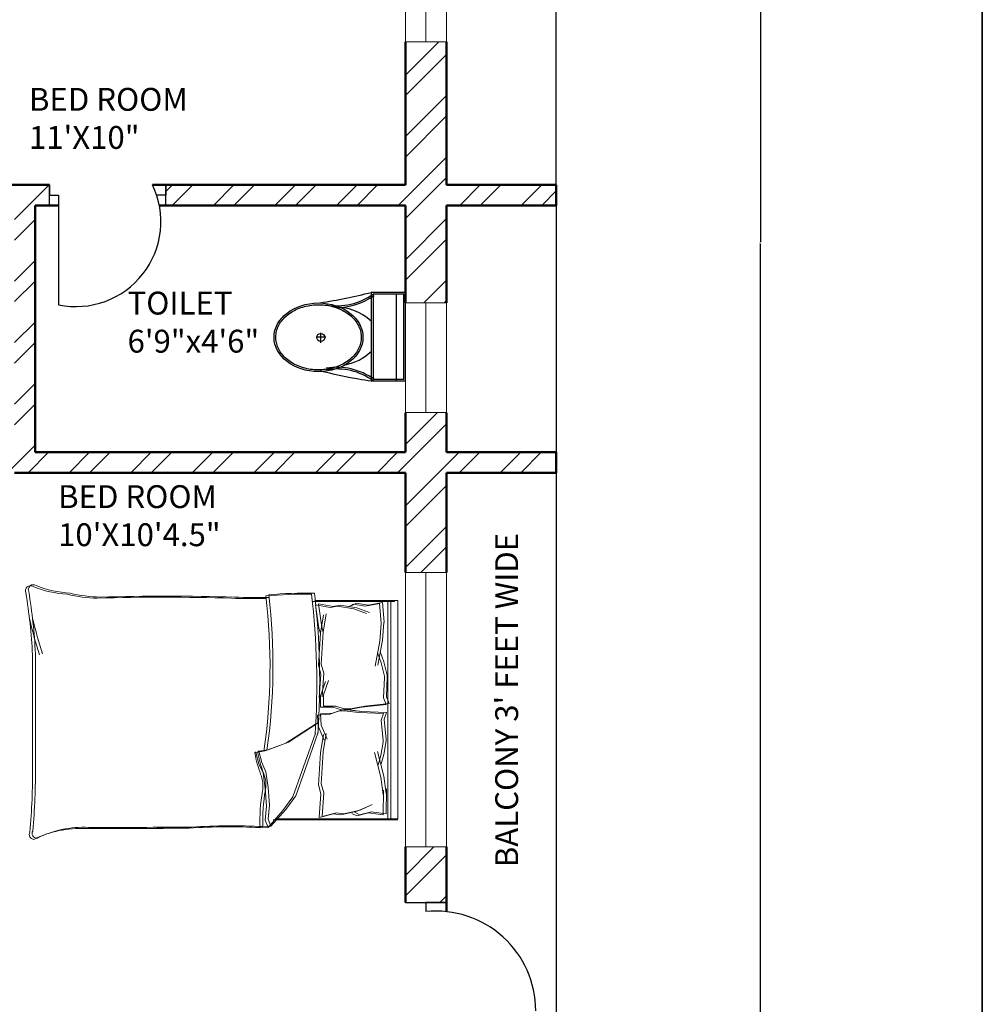
# Model space of a CAD drawing. Units: inches. Extents: x 1980 to 2738, y 1471 to 2568.
# Tile 21 of 22: x 2528 to 2738, y 2112 to 2328. Entities that reach past the tile are written whole.
import ezdxf

# ---------------------------------------------------------------- set-up
doc = ezdxf.new("R2010")
doc.units = ezdxf.units.IN
for name, color, linetype, lineweight in [('A-ANNO-DIMS', 2, 'Continuous', 18), ('A-ANNO-TTLB', 7, 'Continuous', 35), ('A-AREA-IDEN', 7, 'Continuous', 18), ('A-DOOR', 31, 'Continuous', 25), ('A-FLOR-BALC', 7, 'Continuous', 25), ('A-FLOR-FIXT', 8, 'Continuous', 25), ('A-FURN', 8, 'Continuous', 18), ('A-GLAZ', 141, 'Continuous', 18), ('A-WALL', 7, 'Continuous', 50)]:
    doc.layers.add(name, color=color, linetype=linetype, lineweight=lineweight)
doc.layers.add('A-WALL-PATT', color=9, linetype='Continuous', lineweight=13, true_color=0xd19cc7)
doc.styles.get("Standard").update_dxf_attribs({"font": 'arial.ttf'})
doc.dimstyles.get("Standard").update_dxf_attribs({"dimtxt": 0.18, "dimasz": 0.18, "dimexe": 0.18, "dimexo": 0.0625, "dimgap": 0.09, "dimtad": 0, "dimtih": 1, "dimtoh": 1, "dimdec": 4, "dimzin": 0, "dimdsep": 46, "dimtxsty": 'Standard', "dimcen": 0.09, "dimadec": 0, "dimazin": 0, "dimtfac": 1, "dimtdec": 4, "dimtofl": 0, "dimtmove": 0, "dimatfit": 3, "dimfxl": 1, "dimtolj": 1, "dimtzin": 0, "dimarcsym": 0})

# ---------------------------------------------------------------- blocks, each defined once
blk = doc.blocks.new('A$C31115884')
for p, q in [((257.5, 466.4), (257.5, 523.2)), ((283.1, 497.7), (223.4, 497.7)), ((0, 200), (0, 0)), ((520, 200), (0, 200)), ((10, 190), (10, 10)), ((510, 190), (10, 190)), ((510, 10), (510, 190)), ((520, 0), (520, 200)), ((510, 54.5), (0, 54.5)), ((10, 10), (510, 10)), ((0, 0), (520, 0))]:
    blk.add_line(p, q)
blk.add_circle((255.6, 496.4), 23.6)
for centre, radius, start, end in [((2777.7, -204.6), 2807, 165.4549, 171.71327), ((-294.5, 403.3), 364.7, 324.20913, 9.34987), ((-294.5, 403.3), 374.7, 324.20913, 9.34987), ((805.8, 403.3), 364.7, 170.65013, 215.79087), ((3237, 905), 2807, 188.28673, 194.5451), ((139.5, 406.2), 293.5, 315.84364, 2.65635), ((805.8, 403.3), 374.7, 179.20365, 215.79087), ((383.6, 406.2), 293.5, 190.27735, 224.15636)]:
    blk.add_arc(centre, radius, start, end)
blk.add_ellipse((256.2, 509.9), major_axis=(0, -260.7), ratio=0.772727)
blk.add_open_spline([(256.2, 259.2), (263.1, 259.2), (270, 259.7), (287.8, 262.3), (298.7, 265.1), (319.9, 273.1), (330.2, 278.4), (350.1, 291.1), (359.7, 298.7), (377.7, 315.9), (386.2, 325.5), (401.7, 346.6), (408.8, 358.1), (421.3, 382.5), (426.8, 395.5), (435.9, 422.4), (439.5, 436.4), (444.8, 465.1), (446.5, 479.7), (447.9, 509.2), (447.6, 524), (445, 553.3), (442.7, 567.8), (436.3, 596), (432.1, 609.7), (421.9, 636), (416, 648.6), (402.5, 672.1), (395, 683), (378.6, 703), (369.8, 712.1), (351.1, 728), (341.3, 734.8), (320.9, 746.2), (310.4, 750.7), (288.9, 757.3), (278, 759.4), (256, 761), (245, 760.6), (223.1, 757.2), (212.3, 754.3), (191.1, 746.1), (180.8, 740.7), (160.9, 727.8), (151.4, 720.1), (133.5, 702.7), (125.1, 693), (109.6, 671.7), (102.6, 660.2), (90.2, 635.7), (84.9, 622.7), (76, 595.6), (72.4, 581.6), (67.2, 552.9), (65.6, 538.2), (64.4, 508.8), (64.8, 494), (67.5, 464.7), (69.9, 450.2), (76.6, 422), (80.8, 408.3), (91.1, 382.2), (97.2, 369.7), (110.8, 346.3), (118.4, 335.4), (134.8, 315.6), (143.7, 306.7), (162.4, 290.9), (172.3, 284.2), (192.8, 273), (203.3, 268.6), (224.8, 262.2), (235.8, 260.2), (249.9, 259.3), (253, 259.2), (256.2, 259.2)], degree=3, knots=[0, 0, 0, 0, 0.110105, 0.110105, 0.285049, 0.285049, 0.459994, 0.459994, 0.634938, 0.634938, 0.809882, 0.809882, 0.984827, 0.984827, 1.159771, 1.159771, 1.334715, 1.334715, 1.50966, 1.50966, 1.684604, 1.684604, 1.859549, 1.859549, 2.034493, 2.034493, 2.209437, 2.209437, 2.384382, 2.384382, 2.559326, 2.559326, 2.73427, 2.73427, 2.909215, 2.909215, 3.084159, 3.084159, 3.259103, 3.259103, 3.434048, 3.434048, 3.608992, 3.608992, 3.783936, 3.783936, 3.958881, 3.958881, 4.133825, 4.133825, 4.30877, 4.30877, 4.483714, 4.483714, 4.658658, 4.658658, 4.833603, 4.833603, 5.008547, 5.008547, 5.183491, 5.183491, 5.358436, 5.358436, 5.53338, 5.53338, 5.708324, 5.708324, 5.883269, 5.883269, 6.058213, 6.058213, 6.233158, 6.233158, 6.283185, 6.283185, 6.283185, 6.283185])
blk = doc.blocks.new('BED-DOUBLE')
for p, q in [((27.75, 52.87), (24.5, 49.16)), ((27.75, 52.87), (24.5, 49.16)), ((28.38, 53.1), (25.13, 49.39)), ((28.38, 53.1), (25.13, 49.39)), ((29.49, 52.95), (27.75, 52.87, 3.87)), ((29.49, 52.95), (27.75, 52.87, 3.87)), ((28.36, 51.33), (27.75, 52.87)), ((28.36, 51.33), (27.75, 52.87)), ((30.13, 53.18), (28.38, 53.1, 3.87)), ((30.13, 53.18), (28.38, 53.1, 3.87)), ((29, 51.56), (28.38, 53.1)), ((29, 51.56), (28.38, 53.1)), ((0, 51.49), (0.64, 51.49)), ((0, 51.27), (26.61, 51.27)), ((0, 51.27), (26.61, 51.27)), ((0, 51.27), (0, 3.48)), ((0.64, 51.49), (27.25, 51.49)), ((0.64, 51.49), (27.25, 51.49)), ((1.53, 3.48), (1.53, 51.27)), ((1.53, 3.48), (1.53, 51.27)), ((2.17, 3.7), (2.17, 51.49)), ((2.17, 3.7), (2.17, 51.49)), ((2.56, 50.11), (2.46, 44.71)), ((2.56, 50.11), (2.46, 44.71)), ((2.56, 50.11), (5.77, 49.73)), ((2.56, 50.11), (5.77, 49.73)), ((3.2, 50.34), (3.1, 44.94)), ((3.2, 50.34), (3.1, 44.94)), ((3.2, 50.34), (6.41, 49.96)), ((3.2, 50.34), (6.41, 49.96)), ((5.77, 49.73), (8.34, 50.33)), ((5.77, 49.73), (8.34, 50.33)), ((6.41, 49.96), (8.98, 50.56)), ((6.41, 49.96), (8.98, 50.56)), ((11.83, 50.11), (8.26, 49.31)), ((11.83, 50.11), (8.26, 49.31)), ((8.34, 50.33), (9.38, 49.81)), ((8.34, 50.33), (9.38, 49.81)), ((12.47, 50.34), (8.9, 49.54)), ((12.47, 50.34), (8.9, 49.54)), ((8.98, 50.56), (10.02, 50.04)), ((8.98, 50.56), (10.02, 50.04)), ((13.43, 49.92), (11.83, 50.11)), ((13.43, 49.92), (11.83, 50.11)), ((14.07, 50.15), (12.47, 50.34)), ((14.07, 50.15), (12.47, 50.34)), ((16.57, 50.7), (13.43, 49.92)), ((16.57, 50.7), (13.43, 49.92)), ((17.21, 50.93), (14.07, 50.15)), ((17.21, 50.93), (14.07, 50.15)), ((16.17, 45.57), (16.57, 50.7)), ((16.17, 45.57), (16.57, 50.7)), ((16.81, 45.8), (17.21, 50.93)), ((16.81, 45.79), (17.21, 50.93)), ((28.06, 48.23), (28.36, 51.33)), ((28.06, 48.23), (28.36, 51.33)), ((28.69, 48.46), (29, 51.56)), ((28.69, 48.46), (29, 51.56)), ((8.26, 49.31), (5.58, 48.13)), ((8.26, 49.31), (5.58, 48.13)), ((8.9, 49.54), (6.22, 48.36)), ((8.9, 49.54), (6.22, 48.36)), ((24.5, 49.16), (22.33, 46.22)), ((24.5, 49.16), (22.33, 46.22)), ((25.13, 49.39), (22.97, 46.45)), ((25.13, 49.39), (22.97, 46.45)), ((28.36, 44.36), (28.06, 48.23)), ((28.36, 44.36), (28.06, 48.23)), ((29, 44.59), (28.69, 48.46)), ((29, 44.59), (28.69, 48.46)), ((2.46, 44.71), (2.54, 45.71)), ((2.46, 44.71), (2.54, 45.71)), ((2.54, 45.71), (3.07, 41.91)), ((2.54, 45.71), (3.07, 41.91)), ((3.1, 44.94), (3.18, 45.94)), ((3.1, 44.94), (3.18, 45.94)), ((3.18, 45.94), (3.71, 42.14)), ((3.18, 45.94), (3.71, 42.14)), ((16.73, 43.61), (16.17, 45.57)), ((16.73, 43.61), (16.17, 45.57)), ((17.37, 43.83), (16.81, 45.8)), ((17.37, 43.83), (16.81, 45.79)), ((22.33, 46.22), (20.32, 40.64)), ((22.33, 46.22), (20.32, 40.64)), ((22.97, 46.45), (20.96, 40.87)), ((22.97, 46.45), (20.96, 40.87)), ((16.29, 36.6), (16.73, 43.61)), ((16.29, 36.6), (16.73, 43.61)), ((16.93, 36.82), (17.37, 43.83)), ((16.93, 36.82), (17.37, 43.83)), ((28.83, 40.95), (28.36, 44.36)), ((28.83, 40.95), (28.36, 44.36)), ((29.47, 41.18), (29, 44.59)), ((29.47, 41.18), (29, 44.59)), ((3.07, 41.91), (4.42, 36.5)), ((3.07, 41.91), (4.42, 36.5)), ((3.71, 42.14), (5.06, 36.72)), ((3.71, 42.14), (5.06, 36.72)), ((29.76, 38.94), (28.83, 40.95)), ((29.76, 38.94), (28.83, 40.95)), ((30.4, 39.17), (29.47, 41.18)), ((30.4, 39.17), (29.47, 41.18)), ((3.67, 39.2), (3.08, 37.14)), ((3.67, 39.2), (3.08, 37.14)), ((4.31, 39.43), (3.72, 37.36)), ((4.31, 39.43), (3.72, 37.36)), ((20.32, 40.64), (17.38, 32.31)), ((20.32, 40.64), (17.38, 32.31)), ((20.96, 40.87), (18.02, 32.53)), ((20.96, 40.87), (18.02, 32.53)), ((30.38, 36.46), (29.76, 38.94)), ((30.38, 36.46), (29.76, 38.94)), ((31.02, 36.69), (30.4, 39.17)), ((31.02, 36.69), (30.4, 39.17)), ((79.24, 15.06), (79.24, 39.68)), ((79.24, 15.06), (79.24, 39.68)), ((79.88, 15.29), (79.88, 39.91)), ((79.88, 15.29), (79.88, 39.91)), ((3.08, 37.14), (2.54, 34.2)), ((3.08, 37.14), (2.54, 34.2)), ((3.72, 37.36), (3.18, 34.43)), ((3.72, 37.36), (3.18, 34.43)), ((16.27, 32.79), (16.93, 36.82)), ((16.27, 32.79), (16.93, 36.82)), ((29, 36.38), (31.02, 36.69)), ((29, 36.38), (31.02, 36.69)), ((15.63, 32.56), (16.29, 36.6)), ((15.63, 32.56), (16.29, 36.6)), ((18.02, 30.49), (24.52, 34.68)), ((18.02, 30.49), (24.52, 34.68)), ((23.88, 34.45), (28.36, 36.15)), ((23.88, 34.45), (28.36, 36.15)), ((24.52, 34.68), (29, 36.38)), ((24.52, 34.68), (29, 36.38)), ((28.36, 36.15), (30.38, 36.46)), ((28.36, 36.15), (30.38, 36.46)), ((2.54, 34.2), (2.56, 33.88)), ((2.54, 34.2), (2.56, 33.88)), ((2.56, 33.88), (2.98, 29.46)), ((2.56, 33.88), (2.98, 29.46)), ((3.18, 34.43), (3.2, 34.11)), ((3.18, 34.43), (3.2, 34.11)), ((3.2, 34.11), (3.62, 29.68)), ((3.2, 34.11), (3.62, 29.68)), ((16.74, 30.75), (15.45, 33.82)), ((16.74, 30.75), (15.45, 33.82)), ((17.38, 30.98), (16.09, 34.05)), ((17.38, 30.98), (16.09, 34.05)), ((17.38, 30.26), (23.88, 34.45)), ((17.38, 30.26), (23.88, 34.45)), ((16.89, 28.3), (16.74, 30.75)), ((16.89, 28.3), (16.74, 30.75)), ((17.53, 28.53), (17.38, 30.98)), ((17.53, 28.53), (17.38, 30.98)), ((2.98, 29.46), (2.49, 27.98)), ((2.98, 29.46), (2.49, 27.98)), ((3.62, 29.68), (3.13, 28.21)), ((3.62, 29.68), (3.13, 28.21)), ((3.13, 28.21), (8.51, 27.96)), ((3.13, 28.21), (8.51, 27.96)), ((12.38, 27.44), (14.22, 28.13)), ((12.38, 27.44), (14.22, 28.13)), ((13.02, 27.66), (14.86, 28.36)), ((13.02, 27.66), (14.86, 28.36)), ((14.22, 28.13), (16.89, 28.3)), ((14.22, 28.13), (16.89, 28.3)), ((14.86, 28.36), (17.53, 28.53)), ((14.86, 28.36), (17.53, 28.53)), ((1.87, 25.98), (7.22, 26.56)), ((1.87, 25.98), (7.22, 26.56)), ((2.45, 24.54), (1.87, 25.98)), ((2.45, 24.54), (1.87, 25.98)), ((2.49, 27.98), (7.87, 27.73)), ((2.49, 27.98), (7.87, 27.73)), ((2.51, 26.21), (7.86, 26.79)), ((2.51, 26.21), (7.86, 26.79)), ((3.09, 24.77), (2.51, 26.21)), ((3.09, 24.77), (2.51, 26.21)), ((7.22, 26.56), (10.4, 27.14)), ((7.22, 26.56), (10.4, 27.14)), ((7.86, 26.79), (11.04, 27.37)), ((7.86, 26.79), (11.04, 27.37)), ((7.87, 27.73), (11.08, 27.36)), ((7.87, 27.73), (11.08, 27.35)), ((8.51, 27.96), (11.72, 27.58)), ((8.51, 27.96), (11.72, 27.58)), ((10.4, 27.14), (11.7, 27.14)), ((10.4, 27.14), (11.7, 27.14)), ((11.04, 27.37), (12.34, 27.37)), ((11.04, 27.37), (12.34, 27.37)), ((11.08, 27.36), (12.38, 27.44)), ((11.08, 27.35), (12.38, 27.44)), ((11.7, 27.14), (13.58, 26.56)), ((11.7, 27.14), (13.58, 26.56)), ((11.72, 27.58), (13.02, 27.66)), ((11.72, 27.58), (13.02, 27.66)), ((12.34, 27.37), (14.22, 26.79)), ((12.34, 27.37), (14.22, 26.79)), ((13.58, 26.56), (16.26, 26.56)), ((13.58, 26.56), (16.26, 26.56)), ((14.22, 26.79), (16.9, 26.79)), ((14.22, 26.79), (16.9, 26.79)), ((16.26, 26.56), (16.26, 24.1)), ((16.26, 26.56), (16.26, 24.1)), ((16.9, 26.79), (16.9, 24.33)), ((16.9, 26.79), (16.9, 24.33)), ((2.3, 20.09), (2.45, 24.54)), ((2.3, 20.09), (2.45, 24.54)), ((2.94, 20.32), (3.09, 24.77)), ((2.94, 20.32), (3.09, 24.77)), ((16.26, 24.1), (15.17, 20.96)), ((16.26, 24.1), (15.17, 20.96)), ((16.9, 24.33), (15.81, 21.19)), ((16.9, 24.33), (15.81, 21.19)), ((16.17, 19.38), (16.57, 24.52)), ((16.17, 19.38), (16.57, 24.52)), ((16.81, 19.61), (17.21, 24.74)), ((16.81, 19.61), (17.21, 24.74)), ((2.3, 19.77), (2.3, 20.09)), ((2.3, 19.77), (2.3, 20.09)), ((3.03, 16.88), (2.3, 19.77)), ((3.03, 16.88), (2.3, 19.77)), ((2.94, 20), (2.94, 20.32)), ((2.94, 20), (2.94, 20.32)), ((3.67, 17.11), (2.94, 20)), ((3.67, 17.11), (2.94, 20)), ((17.37, 17.65), (16.81, 19.61)), ((17.37, 17.65), (16.81, 19.61)), ((3.32, 12.11), (4.33, 17.6)), ((3.32, 12.11), (4.33, 17.6)), ((3.96, 12.34), (4.97, 17.83)), ((3.96, 12.34), (4.97, 17.83)), ((16.73, 17.42), (16.17, 19.38)), ((16.73, 17.42), (16.17, 19.38)), ((16.29, 10.41), (16.73, 17.42)), ((16.29, 10.41), (16.73, 17.42)), ((16.93, 10.64), (17.37, 17.65)), ((16.93, 10.64), (17.37, 17.65)), ((3.75, 14.86), (3.03, 16.88)), ((3.75, 14.85), (3.03, 16.88)), ((4.39, 15.08), (3.67, 17.11)), ((4.39, 15.08), (3.67, 17.11)), ((3.03, 8.29), (3.32, 12.11)), ((3.03, 8.28), (3.32, 12.11)), ((3.67, 8.51), (3.96, 12.34)), ((3.67, 8.51), (3.96, 12.34)), ((15.63, 6.38), (16.29, 10.41)), ((15.63, 6.38), (16.29, 10.41)), ((16.27, 6.61), (16.93, 10.64)), ((16.27, 6.61), (16.93, 10.64)), ((16.29, 10.41), (16.62, 9.28)), ((16.29, 10.41), (16.62, 9.28)), ((16.62, 9.28), (17.34, 4.18)), ((16.62, 9.28), (17.34, 4.18)), ((16.93, 10.64), (17.26, 9.51)), ((16.93, 10.64), (17.26, 9.51)), ((17.26, 9.51), (17.98, 4.41)), ((17.26, 9.51), (17.98, 4.41)), ((3.01, 8.18), (3.03, 8.29)), ((3.01, 8.18), (3.03, 8.28)), ((3.34, 3.9), (3.01, 8.18)), ((3.34, 3.9), (3.01, 8.18)), ((3.65, 8.41), (3.67, 8.51)), ((3.65, 8.41), (3.67, 8.51)), ((3.98, 4.13), (3.65, 8.41)), ((3.98, 4.13), (3.65, 8.41)), ((3.32, 3.89), (6.5, 4.47)), ((3.32, 3.89), (6.5, 4.47)), ((3.96, 4.12), (7.14, 4.7)), ((3.96, 4.12), (7.14, 4.7)), ((8.95, 5.05), (6.21, 6.06)), ((8.95, 5.05), (6.21, 6.06)), ((6.5, 4.47), (9.1, 4.04)), ((6.5, 4.47), (9.1, 4.04)), ((9.59, 5.28), (6.85, 6.29)), ((9.59, 5.28), (6.85, 6.29)), ((7.14, 4.7), (9.74, 4.27)), ((7.14, 4.7), (9.74, 4.27)), ((12.57, 4.47), (8.95, 5.05)), ((12.57, 4.47), (8.95, 5.05)), ((9.1, 4.04), (10.11, 4.62)), ((9.1, 4.04), (10.11, 4.62)), ((13.21, 4.7), (9.59, 5.28)), ((13.21, 4.7), (9.59, 5.28)), ((9.74, 4.27), (10.75, 4.85)), ((9.74, 4.27), (10.75, 4.85)), ((14.16, 4.76), (12.57, 4.47)), ((14.16, 4.76), (12.57, 4.47)), ((14.8, 4.99), (13.21, 4.7)), ((14.8, 4.99), (13.21, 4.7)), ((17.34, 4.18), (14.16, 4.76)), ((17.34, 4.18), (14.16, 4.76)), ((17.98, 4.41), (14.8, 4.99)), ((17.98, 4.41), (14.8, 4.99)), ((18.11, 3.48), (0, 3.48)), ((18.11, 3.48), (0, 3.48)), ((18.75, 3.7), (0.64, 3.7)), ((18.75, 3.7), (0.64, 3.7))]:
    blk.add_line(p, q)
for centre, radius, start, end in [((68.67, 76.16), 23.07, 267.4714, 296.4681), ((68.67, 76.16), 23.07, 267.4714, 296.4681), ((69.31, 76.39), 23.07, 267.4714, 296.4681), ((69.31, 76.39), 23.07, 267.4714, 296.4681), ((78.87, 54.41), 1.1, 332.6588, 86.02), ((78.87, 54.41), 1.1, 332.6588, 86.02), ((212.28, 41.15), 133.04, 174.4998, 180.6351), ((212.28, 41.15), 133.04, 174.4998, 180.6351), ((79.51, 54.64), 1.1, 332.6588, 86.02), ((79.51, 54.64), 1.1, 332.6588, 86.02), ((212.92, 41.38), 133.04, 174.4998, 180.6351), ((212.92, 41.38), 133.04, 174.4998, 180.6351), ((-6.66, 51.33), 36.18, 349.8763, 2.5657), ((-6.66, 51.33), 36.18, 349.8763, 2.5657), ((36.31, 182.27), 129.5, 266.9791, 273.8365), ((36.31, 182.27), 129.5, 266.9791, 273.8365), ((-6.02, 51.56), 36.18, 349.8763, 2.5657), ((-6.02, 51.56), 36.18, 349.8763, 2.5657), ((36.95, 182.49), 129.5, 266.9791, 273.8365), ((36.95, 182.49), 129.5, 266.9791, 273.8365), ((67.82, -4508.74), 4561.86, 90.00217, 90.28689), ((67.82, -4508.74), 4561.86, 90.00217, 90.28689), ((68.46, -4508.51), 4561.86, 90.00217, 90.28689), ((68.46, -4508.52), 4561.86, 90.00217, 90.28689), ((35.07, 43.74), 6.22, 168.6608, 203.7384), ((35.07, 43.74), 6.22, 168.6608, 203.7384), ((35.71, 43.97), 6.22, 168.6608, 203.7384), ((35.71, 43.97), 6.22, 168.6608, 203.7384), ((1.48, 31.15), 29.65, 10.6617, 19.8806), ((1.48, 31.15), 29.65, 10.6617, 19.8806), ((2.12, 31.38), 29.65, 10.6617, 19.8806), ((2.12, 31.38), 29.65, 10.6617, 19.8806), ((30.44, 36.64), 0.185, 250.2464, 1.1377), ((30.44, 36.64), 0.185, 250.2464, 1.1377), ((31.08, 36.86), 0.185, 250.2464, 1.1377), ((31.08, 36.86), 0.185, 250.2464, 1.1377), ((156.32, 17.76), 129.02, 171.7845, 186.9006), ((156.32, 17.76), 129.02, 171.7845, 186.9006), ((156.96, 17.98), 129.02, 171.7845, 186.9006), ((156.96, 17.98), 129.02, 171.7845, 186.9006), ((182.05, 21.36), 164.97, 176.0865, 186.7821), ((182.05, 21.36), 164.97, 176.0865, 186.7821), ((182.69, 21.59), 164.97, 176.0865, 186.7821), ((182.69, 21.59), 164.97, 176.0865, 186.7821), ((-23.71, -17.22), 106.46, 13.3832, 17.7053), ((-23.71, -17.22), 106.46, 13.3832, 17.7053), ((-23.07, -16.99), 106.46, 13.3832, 17.7053), ((-23.07, -16.99), 106.46, 13.3832, 17.7053), ((201.48, 21.66), 121.76, 182.9958, 189.4091), ((201.48, 21.66), 121.76, 182.9958, 189.4091), ((200.84, 21.43), 121.76, 182.9958, 189.4091), ((200.84, 21.43), 121.76, 182.9958, 189.4091), ((20.1, 85.16), 83.31, 268.7218, 275.604), ((20.1, 85.16), 83.31, 268.7218, 275.604), ((20.74, 85.39), 83.31, 268.7218, 275.604), ((20.74, 85.39), 83.31, 268.7218, 275.604), ((31.17, -167.31), 170.11, 88.4762, 91.0082), ((31.17, -167.31), 170.11, 88.4762, 91.0082), ((31.81, -167.08), 170.11, 88.4762, 91.0082), ((31.81, -167.08), 170.11, 88.4762, 91.0082), ((50.61, 484.82), 482.31, 268.2277, 271.7185), ((50.61, 484.82), 482.31, 268.2277, 271.7185), ((51.25, 485.05), 482.31, 268.2277, 271.7185), ((51.25, 485.05), 482.31, 268.2277, 271.7185), ((64.51, -26.9), 29.63, 76.0648, 88.9113), ((64.51, -26.9), 29.63, 76.0648, 88.9113), ((65.15, -26.67), 29.63, 76.0648, 88.9113), ((65.15, -26.67), 29.63, 76.0648, 88.9113), ((70.28, -21.66), 23.56, 67.9751, 86.652), ((70.28, -21.66), 23.56, 67.9751, 86.652), ((70.91, -21.43), 23.56, 67.9751, 86.652), ((70.91, -21.43), 23.56, 67.9751, 86.652), ((79.72, 1.09), 1.09, 236.1736, 23.4781), ((79.72, 1.09), 1.09, 236.1736, 23.4781), ((80.36, 1.32), 1.09, 236.1736, 23.4781), ((80.36, 1.32), 1.09, 236.1736, 23.4781)]:
    blk.add_arc(centre, radius, start, end)
blk = doc.blocks.new('WIN-60IN-WALL')
for p, q in [((0, 9), (0, 0)), ((60, 9), (0, 9)), ((60, 4.5), (60, 9)), ((60, 9), (60, 0)), ((0, 0), (0, 4.5)), ((0, 4.5), (60, 4.5)), ((0, 0), (60, 0))]:
    blk.add_line(p, q)
blk = doc.blocks.new('WIN-24IN-WALL')
for p, q in [((4.5, 24), (0, 24)), ((0, 24), (9, 24)), ((0, 24), (0, 0)), ((4.5, 0), (4.5, 24)), ((9, 0), (9, 24)), ((0, 0), (9, 0)), ((9, 0), (4.5, 0))]:
    blk.add_line(p, q)
blk = doc.blocks.new('*D35')
at = {"layer": 'A-ANNO-DIMS', "color": 0, "lineweight": -2, "transparency": 16777216}
for p, q in [((2081.08, 2291.77), (2081.08, 2507.54)), ((2081.26, 2507.36), (2362.79, 2507.36)), ((2644.9, 2507.36), (2363.37, 2507.36)), ((2645.08, 2291.77), (2645.08, 2507.54))]:
    blk.add_line(p, q, dxfattribs=at)
at = {"layer": 'A-ANNO-DIMS', "color": 0, "transparency": 16777216}
for points in [[(2081.26, 2507.39), (2081.26, 2507.33), (2081.08, 2507.36)], [(2644.9, 2507.39), (2644.9, 2507.33), (2645.08, 2507.36)]]:
    blk.add_solid(points, dxfattribs=at)
at = {"layer": 'Defpoints', "color": 0, "transparency": 16777216}
for p in [(2645.08, 2507.36), (2081.08, 2291.71), (2645.08, 2291.71)]:
    blk.add_point(p, dxfattribs=at)
at = {"layer": 'A-ANNO-DIMS', "color": 0, "transparency": 16777216, "insert": (2363.08, 2507.36), "char_height": 0.18, "attachment_point": 5}
blk.add_mtext('\\A1;564', dxfattribs=at)
blk = doc.blocks.new('*D39')
at = {"layer": 'A-ANNO-DIMS', "color": 0, "lineweight": -2, "transparency": 16777216}
for p, q in [((2621.15, 2462.71), (2689.91, 2462.71)), ((2689.73, 2462.53), (2689.73, 2279.14)), ((2689.73, 2095.39), (2689.73, 2278.77)), ((2579.97, 2095.21), (2689.91, 2095.21))]:
    blk.add_line(p, q, dxfattribs=at)
at = {"layer": 'A-ANNO-DIMS', "color": 0, "transparency": 16777216}
for points in [[(2689.7, 2462.53), (2689.76, 2462.53), (2689.73, 2462.71)], [(2689.7, 2095.39), (2689.76, 2095.39), (2689.73, 2095.21)]]:
    blk.add_solid(points, dxfattribs=at)
at = {"layer": 'Defpoints', "color": 0, "transparency": 16777216}
for p in [(2621.08, 2462.71), (2689.73, 2462.71), (2579.9, 2095.21)]:
    blk.add_point(p, dxfattribs=at)
at = {"layer": 'A-ANNO-DIMS', "color": 0, "transparency": 16777216, "insert": (2689.73, 2278.96), "char_height": 0.18, "attachment_point": 5}
blk.add_mtext('\\A1;367.5', dxfattribs=at)

msp = doc.modelspace()

# ---------------------------------------------------------------- hatches: boundary and pattern name
at = {"layer": 'A-WALL-PATT'}
h = msp.add_hatch(dxfattribs=at)
h.set_pattern_fill('ANSI32', color=256)
h.paths.add_polyline_path([(2257.5661, 2416.2064), (2257.5661, 2420.7064), (2250.5833, 2420.7064), (2250.5833, 2462.7064), (2246.0833, 2462.7064), (2246.0833, 2420.7064), (2237.0791, 2420.7064), (2237.0791, 2411.7064), (2246.0833, 2411.7064), (2246.0833, 2291.7064), (2242.6109, 2291.7064), (2242.6109, 2287.2064), (2246.0833, 2287.2064), (2250.5833, 2287.2064), (2250.5833, 2291.7064), (2250.5833, 2411.7064), (2257.5661, 2411.7064)])
h.paths.add_polyline_path([(2387.0396, 2416.2064), (2387.0396, 2420.7064), (2367.5833, 2420.7064), (2367.5833, 2462.7064), (2358.5833, 2462.7064), (2358.5833, 2420.7064), (2329.3087, 2420.7064), (2329.3087, 2411.7064), (2358.5833, 2411.7064), (2358.5833, 2321.7275), (2358.5833, 2309.7064), (2347.3089, 2309.7064), (2293.3089, 2309.7064), (2293.3089, 2259.0771), (2297.8089, 2259.0771), (2297.8089, 2305.2064), (2347.3089, 2305.2064), (2347.3089, 2284.7412), (2351.8089, 2284.7412), (2351.8089, 2305.2064), (2372.3188, 2305.2064), (2372.3761, 2284.3899), (2377.0295, 2284.3899), (2377.0295, 2299.3058), (2377.0295, 2305.2064), (2426.5295, 2305.2064), (2426.5295, 2257.5573), (2431.0295, 2257.5573), (2431.0295, 2309.7064), (2377.0295, 2309.7064), (2367.5833, 2309.7064), (2367.5833, 2321.7275), (2367.5833, 2411.7064), (2387.0396, 2411.7064)])
h.paths.add_polyline_path([(2448.5267, 2416.2064), (2448.5267, 2420.7064), (2423.0396, 2420.7064), (2423.0396, 2411.7064), (2448.5267, 2411.7064)])
h.paths.add_polyline_path([(2130.9128, 2416.2064), (2130.9128, 2420.7064), (2105.0833, 2420.7064), (2105.0833, 2386.6942), (2114.0833, 2386.6942), (2114.0833, 2411.7064), (2130.9128, 2411.7064)])
h.paths.add_polyline_path([(2212.9478, 2420.7064), (2190.9128, 2420.7064), (2190.9128, 2411.7064), (2212.9478, 2411.7064), (2212.9478, 2416.2064)])
h.paths.add_polyline_path([(2114.0833, 2326.6942), (2105.0833, 2326.6942), (2105.0833, 2291.7064), (2081.0833, 2291.7064), (2081.0833, 2287.2064), (2105.0833, 2287.2064), (2105.0833, 2276.1935), (2114.0833, 2276.1935), (2114.0833, 2287.2064), (2166.3825, 2287.2064), (2166.3825, 2289.4564), (2166.3825, 2291.7064), (2114.0833, 2291.7064)])
h.paths.add_polyline_path([(2114.0833, 2252.1935), (2105.0833, 2252.1935), (2105.0833, 2233.2064), (2081.0833, 2233.2064), (2081.0833, 2228.7064), (2105.0833, 2228.7064), (2105.0833, 2213.4478), (2114.0833, 2213.4478), (2114.0833, 2228.7064), (2195.0833, 2228.7064), (2199.5833, 2228.7064), (2208.4455, 2228.7064), (2208.4455, 2230.9564), (2208.4455, 2233.2064), (2199.5833, 2233.2064), (2199.5833, 2287.2064), (2206.8904, 2287.2064), (2206.8904, 2289.4564), (2206.8904, 2291.7064), (2189.446, 2291.7064), (2189.446, 2289.4564), (2189.446, 2287.2064), (2195.0833, 2287.2064), (2195.0833, 2233.2064), (2114.0833, 2233.2064)])
h.paths.add_polyline_path([(2114.0833, 2153.4478), (2109.5833, 2153.4478), (2105.0833, 2153.4478), (2105.0833, 2135.2374), (2114.0833, 2135.2374)], flags=17)
h.paths.add_polyline_path([(2135.9619, 2095.4081), (2140.1805, 2095.4081), (2140.1805, 2104.2064), (2114.0833, 2104.2064), (2114.0833, 2110.3997), (2109.5833, 2110.3997), (2105.0833, 2110.3997), (2105.0833, 2104.2064), (2081.0833, 2104.2064), (2081.0833, 2099.7064), (2105.0833, 2099.7064), (2127.5416, 2099.8532), (2127.5416, 2056.9393), (2136.2133, 2056.9393)], flags=17)
h.paths.add_polyline_path([(2255.4895, 2104.2064), (2250.5833, 2104.2064), (2250.5833, 2233.2064), (2246.0833, 2233.2064), (2242.4941, 2233.2064), (2242.4941, 2228.7064), (2246.0833, 2228.7064), (2246.0833, 2104.2064), (2163.6825, 2104.2064), (2163.6825, 2099.8072), (2163.6825, 2095.4081), (2191.4325, 2095.4081), (2191.4325, 2011.2064), (2186.0833, 2011.2064), (2136.5143, 2010.8824), (2136.3702, 2032.9403), (2131.9559, 2032.9115), (2127.5416, 2032.8826), (2127.5416, 2006.7064), (2105.0833, 2006.7064), (2081.0833, 2006.7064), (2081.0833, 2002.2064), (2105.0833, 2002.2064), (2105.0833, 1995.9329), (2114.0833, 1995.9329), (2114.0833, 2002.2064), (2246.0833, 2002.2064), (2246.0833, 1877.7064), (2242.1358, 1877.7064), (2242.1358, 1873.2064), (2250.5833, 1873.2064), (2250.5833, 2002.2064), (2255.3335, 2002.2064), (2255.3335, 2011.2064), (2195.9325, 2011.2064), (2195.9325, 2095.2064), (2255.4895, 2095.2064), (2255.4895, 2099.5471)])
h.paths.add_polyline_path([(2199.5833, 1873.2064), (2209.827, 1873.2064), (2209.827, 1875.4564), (2209.827, 1877.7064), (2114.0833, 1877.7064), (2114.0833, 1890.0968), (2105.0833, 1890.0968), (2105.0833, 1877.7064), (2081.0833, 1877.7064), (2081.0833, 1873.2064), (2105.0833, 1873.2064), (2105.0833, 1857.7279), (2114.0833, 1857.7279), (2114.0833, 1873.2064), (2195.0833, 1873.2064), (2195.0833, 1819.2064), (2190.298, 1819.2064), (2190.298, 1814.7064), (2209.8976, 1814.7064), (2209.8976, 1816.9564), (2209.8976, 1819.2064), (2199.5833, 1819.2064)])
h.paths.add_polyline_path([(2114.0833, 1814.7064), (2166.2538, 1814.7064), (2166.2538, 1816.9564), (2166.2538, 1819.2064), (2114.0833, 1819.2064), (2114.0833, 1833.7279), (2109.5833, 1833.7279), (2105.0833, 1833.7279), (2105.0833, 1819.2064), (2081.0833, 1819.2064), (2081.0833, 1814.7064), (2105.0833, 1814.7064), (2105.0833, 1782.5516), (2114.0833, 1782.5516)])
h.paths.add_polyline_path([(2114.0833, 1722.5516), (2109.5833, 1722.5516), (2105.0833, 1722.5516), (2105.0833, 1685.7064), (2124.5104, 1685.7064), (2124.5104, 1690.2064), (2124.5104, 1694.7064), (2114.0833, 1694.7064)])
h.paths.add_polyline_path([(2218.8787, 1694.7064), (2184.5104, 1694.7064), (2184.5104, 1685.7064), (2218.8787, 1685.7064), (2218.8787, 1690.2064)])
h.paths.add_polyline_path([(2250.5833, 1819.2064), (2242.6431, 1819.2064), (2242.6431, 1816.9564), (2242.6431, 1814.7064), (2246.0833, 1814.7064), (2246.0833, 1694.7064), (2240.4035, 1694.7064), (2240.4035, 1690.2064), (2240.4035, 1685.7064), (2246.0833, 1685.7064), (2246.0833, 1643.7064), (2250.5833, 1643.7064), (2250.5833, 1685.7064), (2255.9859, 1685.7064), (2255.9859, 1690.2064), (2255.9859, 1694.7064), (2250.5833, 1694.7064)])
h.paths.add_polyline_path([(2297.4764, 1694.7064), (2279.3934, 1694.7064), (2279.3934, 1690.2064), (2279.3934, 1685.7064), (2297.4764, 1685.7064), (2297.4764, 1690.2064)])
h.paths.add_polyline_path([(2377.1596, 1694.7064), (2367.5833, 1694.7064), (2367.5833, 1787.7064), (2431.0295, 1787.7064), (2431.0295, 1792.2064), (2431.0295, 1849.4149), (2428.7795, 1849.4149), (2426.5295, 1849.4149), (2426.5295, 1792.2064), (2421.5833, 1792.2064), (2367.5833, 1792.2064), (2297.8089, 1792.2064), (2297.8089, 1850.2946), (2295.5589, 1850.2946), (2293.3089, 1850.2946), (2293.3089, 1792.2064), (2293.3089, 1787.7064), (2297.8089, 1787.7064), (2358.5833, 1787.7064), (2358.5833, 1694.7064), (2333.4764, 1694.7064), (2333.4764, 1685.7064), (2358.5833, 1685.7064), (2358.5833, 1643.7064), (2367.5833, 1643.7064), (2367.5833, 1685.7064), (2377.1596, 1685.7064)])
h.paths.add_polyline_path([(2442.4912, 1694.7064), (2413.1596, 1694.7064), (2413.1596, 1685.7064), (2442.4912, 1685.7064)])
h.paths.add_polyline_path([(2480.0833, 1814.7064), (2483.4816, 1814.7064), (2483.4816, 1817.9384), (2483.4816, 1819.2064), (2475.5833, 1819.2064), (2475.5833, 1694.7064), (2470.7283, 1694.7064), (2470.7283, 1685.7064), (2475.5833, 1685.7064), (2475.5833, 1643.7064), (2480.0833, 1643.7064), (2480.0833, 1685.7064), (2486.3293, 1685.7064), (2486.3293, 1690.2064), (2486.3293, 1694.7064), (2480.0833, 1694.7064)])
h.paths.add_polyline_path([(2621.0833, 1721.7349), (2612.0833, 1721.7349), (2612.0833, 1694.7064), (2586.1453, 1694.7064), (2586.1453, 1685.7064), (2621.0833, 1685.7064)])
h.paths.add_polyline_path([(2526.1453, 1690.2064), (2526.1453, 1694.7064), (2511.584, 1694.7064), (2511.584, 1690.2064), (2511.584, 1685.7064), (2526.1453, 1685.7064)])
h.paths.add_polyline_path([(2645.0833, 1819.2064), (2621.0833, 1819.2064), (2621.0833, 1835.8527), (2616.5833, 1835.8527), (2612.0833, 1835.8527), (2612.0833, 1819.2064), (2560.2541, 1819.2064), (2560.2541, 1814.7064), (2612.0833, 1814.7064), (2612.0833, 1781.7349), (2621.0833, 1781.7349), (2621.0833, 1814.7064), (2645.0833, 1814.7064)])
h.paths.add_polyline_path([(2645.0833, 1877.7064), (2621.0833, 1877.7064), (2621.0833, 1886.4375), (2612.0833, 1886.4375), (2612.0833, 1877.7064), (2517.1032, 1877.7064), (2517.1032, 1875.4564), (2517.1032, 1873.2064), (2526.5833, 1873.2064), (2526.5833, 1819.2064), (2516.6454, 1819.2064), (2516.6454, 1816.9564), (2516.6454, 1814.7064), (2536.4445, 1814.7064), (2536.4445, 1816.9564), (2536.4445, 1819.2064), (2531.0833, 1819.2064), (2531.0833, 1873.2064), (2612.0833, 1873.2064), (2612.0833, 1859.8527), (2621.0833, 1859.8527), (2621.0833, 1873.2064), (2645.0833, 1873.2064)])
h.paths.add_polyline_path([(2645.0833, 2006.7064), (2621.0833, 2006.7064), (2588.5085, 2006.7064), (2588.5085, 2052.9125), (2579.9045, 2052.9125), (2579.9045, 2011.2064), (2519.9045, 2011.2064), (2519.9045, 2095.2064), (2553.1204, 2095.2064), (2553.1204, 2104.2064), (2480.0833, 2104.2064), (2480.0833, 2228.7064), (2484.3832, 2228.7064), (2484.3832, 2230.9564), (2484.3832, 2233.2064), (2475.5833, 2233.2064), (2475.5833, 2104.2064), (2463.1308, 2104.2064), (2463.1308, 2095.2064), (2501.2463, 2095.2064), (2510.9045, 2095.2064), (2515.4045, 2095.2064), (2515.4045, 2011.2064), (2510.9045, 2011.2064), (2501.2463, 2011.2064), (2462.5957, 2011.2064), (2462.5957, 2002.2064), (2475.5833, 2002.2064), (2475.5833, 1873.2064), (2483.6146, 1873.2064), (2483.6146, 1875.4564), (2483.6146, 1877.7064), (2480.0833, 1877.7064), (2480.0833, 2002.2064), (2612.0833, 2002.2064), (2612.0833, 1996.309), (2621.0833, 1996.309), (2621.0833, 2002.2064), (2645.0833, 2002.2064)])
h.paths.add_polyline_path([(2588.5085, 2099.7277), (2621.0833, 2099.7277), (2645.0833, 2099.7064), (2645.0833, 2104.2064), (2621.0833, 2104.2064), (2621.0833, 2109.0038), (2616.5833, 2109.0038), (2612.0833, 2109.0038), (2612.0833, 2104.2064), (2575.0621, 2104.2064), (2575.0621, 2099.7064), (2575.0621, 2095.2064), (2579.9045, 2095.2064), (2579.9045, 2076.9125), (2588.5085, 2076.9125)], flags=17)
h.paths.add_polyline_path([(2367.5833, 2002.2064), (2373.7228, 2002.2064), (2373.7228, 2006.7064), (2373.7228, 2011.2064), (2350.7889, 2011.2064), (2350.7889, 2006.7064), (2350.7889, 2002.2064), (2358.5833, 2002.2064), (2358.5833, 1877.7064), (2293.3089, 1877.7064), (2293.3089, 1870.4987), (2297.8089, 1870.4987), (2297.8089, 1873.2064), (2347.3089, 1873.2064), (2347.3089, 1847.2208), (2351.8089, 1847.2208), (2351.8089, 1873.2064), (2372.5295, 1873.2064), (2372.5295, 1847.8619), (2377.0295, 1847.8619), (2377.0295, 1873.2064), (2426.5295, 1873.2064), (2426.5295, 1868.7339), (2431.0295, 1868.7339), (2431.0295, 1877.7064), (2367.5833, 1877.7064)])
h.paths.add_polyline_path([(2531.0833, 2287.2064), (2534.2285, 2287.2064), (2534.2285, 2291.7064), (2516.7886, 2291.7064), (2516.7886, 2287.2064), (2526.5833, 2287.2064), (2526.5833, 2233.2064), (2517.9112, 2233.2064), (2517.9112, 2230.9564), (2517.9112, 2228.7064), (2526.5833, 2228.7064), (2531.0833, 2228.7064), (2612.0833, 2228.7064), (2612.0833, 2206.8504), (2621.0833, 2206.8504), (2621.0833, 2228.7064), (2645.0833, 2228.7064), (2645.0833, 2233.2064), (2621.0833, 2233.2064), (2621.0833, 2241.8536), (2616.5833, 2241.8536), (2612.0833, 2241.8536), (2612.0833, 2233.2064), (2531.0833, 2233.2064)])
h.paths.add_polyline_path([(2645.0833, 2291.7064), (2621.0833, 2291.7064), (2621.0833, 2323.0138), (2616.5833, 2323.0138), (2612.0833, 2323.0138), (2612.0833, 2291.7064), (2559.6852, 2291.7064), (2559.6852, 2289.4564), (2559.6852, 2287.2064), (2612.0833, 2287.2064), (2612.0833, 2265.8536), (2621.0833, 2265.8536), (2621.0833, 2287.2064), (2645.0833, 2287.2064)])
h.paths.add_polyline_path([(2621.0833, 2420.7064), (2582.8189, 2420.7064), (2582.8189, 2411.7064), (2612.0833, 2411.7064), (2612.0833, 2383.0138), (2621.0833, 2383.0138)])
h.paths.add_polyline_path([(2480.0833, 2411.7064), (2485.7342, 2411.7064), (2485.7342, 2416.2064), (2485.7342, 2420.7064), (2480.0833, 2420.7064), (2480.0833, 2462.7064), (2475.5833, 2462.7064), (2475.5833, 2420.7064), (2469.4083, 2420.7064), (2469.4083, 2411.7064), (2475.5833, 2411.7064), (2475.5833, 2291.7064), (2475.5833, 2287.2064), (2482.9195, 2287.2064), (2482.9195, 2289.4564), (2482.9195, 2291.7064), (2480.0833, 2291.7064)])
h.paths.add_polyline_path([(2367.5833, 2228.7064), (2431.0295, 2228.7064), (2431.0295, 2233.2064), (2431.0295, 2237.4203), (2428.7795, 2237.4203), (2426.5295, 2237.4203), (2426.5295, 2233.2064), (2377.0295, 2233.2064), (2377.0295, 2260.3837), (2372.4423, 2260.3837), (2372.517, 2233.2635), (2351.8089, 2233.2064), (2351.8089, 2260.7412), (2347.3089, 2260.7412), (2347.3089, 2233.2064), (2297.8089, 2233.2064), (2297.8089, 2236.9324), (2293.3089, 2236.9324), (2293.3089, 2228.7064), (2358.5833, 2228.7064), (2358.5833, 2104.2064), (2353.3665, 2104.2064), (2353.3665, 2095.2064), (2373.8869, 2095.2064), (2373.8869, 2099.7064), (2373.8869, 2104.2064), (2367.5833, 2104.2064)])
h.paths.add_polyline_path([(2321.2323, 2104.2064), (2303.4895, 2104.2064), (2303.4895, 2095.2064), (2321.2323, 2095.2064), (2321.2323, 2099.7064)], flags=0)
h.paths.add_polyline_path([(2415.1308, 2099.7064), (2415.1308, 2104.2064), (2404.81, 2104.2064), (2404.81, 2095.2064), (2415.1308, 2095.2064)], flags=17)
h.paths.add_polyline_path([(2318.6336, 2011.2064), (2303.3335, 2011.2064), (2303.3335, 2002.2064), (2318.6336, 2002.2064)], flags=0)
h.paths.add_polyline_path([(2414.5957, 2011.2064), (2406.2461, 2011.2064), (2406.2461, 2006.7064), (2406.2461, 2002.2064), (2414.5957, 2002.2064)], flags=17)
h = msp.add_hatch(dxfattribs=at)
h.set_pattern_fill('ANSI32', color=256)
h.paths.add_polyline_path([(2321.2323, 2104.2064), (2303.4895, 2104.2064), (2303.4895, 2095.2064), (2321.2323, 2095.2064), (2321.2323, 2099.7064)])
h.paths.add_polyline_path([(2318.6336, 2011.2064), (2303.3335, 2011.2064), (2303.3335, 2002.2064), (2318.6336, 2002.2064)])
h.paths.add_polyline_path([(2114.0833, 1972.9983), (2109.5833, 1972.9983), (2105.0833, 1972.9983), (2105.0833, 1950.0968), (2114.0833, 1950.0968)])
h.paths.add_polyline_path([(2621.0833, 1971.9446), (2616.5833, 1971.9446), (2612.0833, 1971.9446), (2612.0833, 1946.4375), (2621.0833, 1946.4375)])
h.paths.add_polyline_path([(2621.0833, 2146.8504), (2612.0833, 2146.8504), (2612.0833, 2134.6713), (2621.0833, 2134.6713)])

# ---------------------------------------------------------------- linework, layer by layer
at = {"layer": 'A-ANNO-TTLB'}
msp.add_lwpolyline([(1979.5621, 2567.5568), (2738.2543, 2567.5568), (2738.2543, 1471.317), (1979.5621, 1471.317)], close=True, dxfattribs=at)
at = {"layer": 'A-DOOR'}
for p, q in [((2534.2285, 2287.2064), (2534.2285, 2291.7064)), ((2534.2285, 2291.7064), (2534.2285, 2289.4564)), ((2559.6852, 2287.2064), (2559.6852, 2291.7064)), ((2559.6852, 2291.7064), (2559.6852, 2289.4564)), ((2534.2285, 2289.4564), (2536.2285, 2289.4564)), ((2536.2285, 2289.4564), (2536.2285, 2265.4564)), ((2559.6852, 2289.4564), (2557.6852, 2289.4564)), ((2612.0833, 2134.6713), (2621.0833, 2134.6713)), ((2621.0833, 2134.6713), (2616.5833, 2134.6713)), ((2616.5833, 2134.6713), (2616.5833, 2132.6713))]:
    msp.add_line(p, q, dxfattribs=at)
for centre, radius, start, end in [((2540.0097, 2283.6674), 18.5994, 258.269954, 25.608709), ((2618.8024, 2111.0038), 21.7809, 360, 95.847634)]:
    msp.add_arc(centre, radius, start, end, dxfattribs=at)
at = {"layer": 'A-FLOR-BALC'}
msp.add_line((2645.0833, 2287.2064), (2645.0833, 1819.2064), dxfattribs=at)
at = {"layer": 'A-GLAZ'}
msp.add_line((2621.0833, 2241.8536), (2621.0833, 2241.8536), dxfattribs=at)
at = {"layer": 'A-WALL'}
for p, q in [((2612.0833, 2323.0138), (2612.0833, 2291.7064)), ((2621.0833, 2323.0138), (2621.0833, 2291.7064)), ((2515.1245, 2291.7064), (2534.2285, 2291.7064)), ((2556.782, 2291.7064), (2612.0833, 2291.7064)), ((2612.0833, 2291.7064), (2612.0833, 2291.7064)), ((2621.0833, 2291.7064), (2645.0833, 2291.7064)), ((2645.0833, 2291.7064), (2645.0833, 2287.2064)), ((2531.0833, 2287.2064), (2531.0833, 2233.2064)), ((2531.0833, 2287.2064), (2536.2285, 2287.2064)), ((2536.2285, 2287.2064), (2531.0833, 2287.2064)), ((2612.0833, 2287.2064), (2558.2693, 2287.2064)), ((2558.2693, 2287.2064), (2612.0833, 2287.2064)), ((2612.0833, 2287.2064), (2612.0833, 2265.8536)), ((2612.0833, 2287.2064), (2612.0833, 2287.2064)), ((2645.0833, 2287.2064), (2621.0833, 2287.2064)), ((2621.0833, 2287.2064), (2621.0833, 2265.8536)), ((2612.0833, 2241.8536), (2612.0833, 2233.2064)), ((2621.0833, 2241.8536), (2621.0833, 2233.2064)), ((2531.0833, 2233.2064), (2612.0833, 2233.2064)), ((2531.0833, 2233.2064), (2531.0833, 2233.2064)), ((2645.0833, 2233.2064), (2621.0833, 2233.2064)), ((2645.0833, 2228.7064), (2645.0833, 2233.2064)), ((2531.0833, 2228.7064), (2526.5833, 2228.7064)), ((2612.0833, 2228.7064), (2531.0833, 2228.7064)), ((2612.0833, 2228.7064), (2612.0833, 2206.8504)), ((2621.0833, 2228.7064), (2645.0833, 2228.7064)), ((2621.0833, 2228.7064), (2621.0833, 2206.8504)), ((2612.0833, 2146.8504), (2612.0833, 2134.6713)), ((2621.0833, 2146.8504), (2621.0833, 2132.6649))]:
    msp.add_line(p, q, dxfattribs=at)

# ---------------------------------------------------------------- block references
at = {"layer": 'A-FLOR-FIXT', "xscale": 0.0372717239612423, "yscale": 0.0372717239612423, "zscale": 0.0372717239612423, "rotation": 89.99999999999999}
msp.add_blockref('A$C31115884', (2612.0833, 2248.7977), dxfattribs=at)
at = {"layer": 'A-FURN', "rotation": 180}
msp.add_blockref('BED-DOUBLE', (2610.4165, 2204.2206), dxfattribs=at)
at = {"layer": 'A-GLAZ', "rotation": 270}
msp.add_blockref('WIN-60IN-WALL', (2612.0828, 2383.0136), dxfattribs=at)
at = {"layer": 'A-GLAZ'}
msp.add_blockref('WIN-24IN-WALL', (2612.083, 2241.854), dxfattribs=at)
at = {"layer": 'A-GLAZ', "extrusion": (0, 0, -1), "zscale": -1, "rotation": 90}
msp.add_blockref('WIN-60IN-WALL', (-2612.0828, 2146.8506), dxfattribs=at)

# ---------------------------------------------------------------- texts
at = {"layer": 'A-AREA-IDEN', "char_height": 5, "attachment_point": 1}
for s, width, insert in [('BED ROOM\\P11\'X10"', 124.385019, (2529.7503, 2312.9105)), ('TOILET\\P6\'9"x4\'6"', 102.310849, (2551.3147, 2268.327)), ('BED ROOM\\P10\'X10\'4.5"', 182.009382, (2536.1265, 2225.9797))]:
    msp.add_mtext_dynamic_manual_height_columns(s, width=width, gutter_width=12.5, heights=[0], dxfattribs=dict(at, insert=insert))
at = {"layer": 'A-AREA-IDEN', "insert": (2631.7303, 2142.3953), "char_height": 5, "attachment_point": 1, "rotation": 90}
msp.add_mtext_dynamic_manual_height_columns("BALCONY 3' FEET WIDE", width=174.780251, gutter_width=12.5, heights=[0], dxfattribs=at)

# ---------------------------------------------------------------- dimensions: what is measured, and where the dimension line sits
at = {"layer": 'A-ANNO-DIMS'}
dim = msp.add_linear_dim(base=(2645.0833, 2507.3564), p1=(2081.0833, 2291.7064), p2=(2645.0833, 2291.7064), dimstyle='Standard', override={"dimdec": 0, "dimlfac": 1, "dimrnd": 0, "dimzin": 0, "dimdsep": 46, "dimlunit": 2}, dxfattribs=at)
dim.commit()
dim.dimension.update_dxf_attribs({"geometry": '*D35', "text_midpoint": (2363.0833, 2507.3564)})
dim = msp.add_linear_dim(base=(2689.7333, 2462.7064), p1=(2579.9045, 2095.2064), p2=(2621.0833, 2462.7064), angle=90, dimstyle='Standard', override={"dimdec": 1, "dimlfac": 1, "dimrnd": 0, "dimzin": 0, "dimdsep": 46, "dimlunit": 2}, dxfattribs=at)
dim.commit()
dim.dimension.update_dxf_attribs({"geometry": '*D39', "text_midpoint": (2689.7333, 2278.9564)})

doc.saveas('drawing.dxf')
